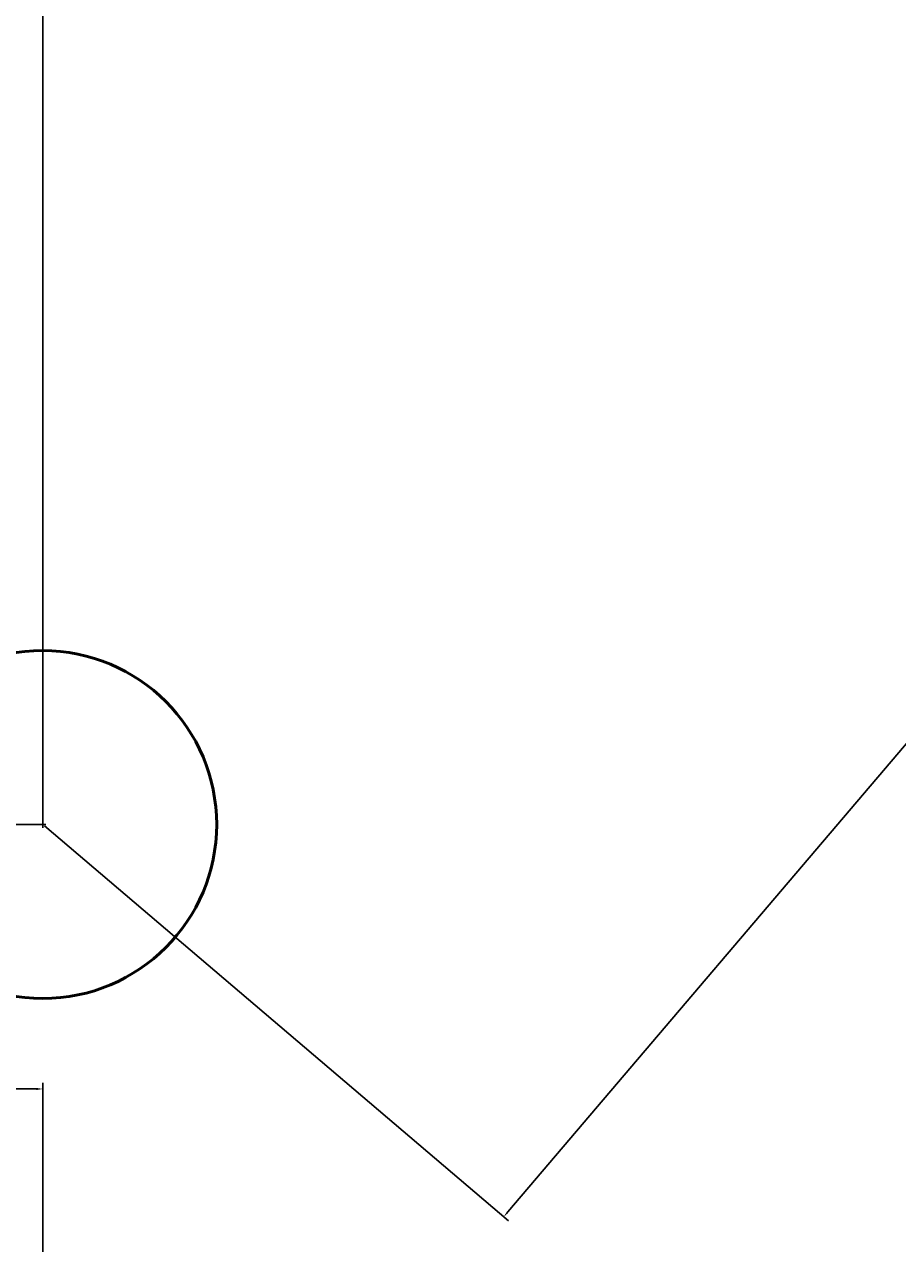
# Model space of a CAD drawing. Units: inches. Extents: x 457 to 775, y 319 to 541.
# Tile 4 of 12: x 554 to 580, y 350 to 385. Entities that reach past the tile are written whole.
import ezdxf

# ---------------------------------------------------------------- set-up
doc = ezdxf.new("R2010")
doc.units = ezdxf.units.IN
doc.header["$MEASUREMENT"] = 0
doc.layers.add('M-DIMS', color=2, linetype='Continuous', lineweight=18)
doc.layers.add('M-OUTL', color=7, linetype='Continuous', lineweight=50)
doc.styles.get("Standard").update_dxf_attribs({"font": 'arial.ttf'})
doc.dimstyles.get("Standard").update_dxf_attribs({"dimtxt": 0.18, "dimasz": 0.18, "dimexe": 0.18, "dimexo": 0.0625, "dimgap": 0.09, "dimtad": 0, "dimtih": 1, "dimtoh": 1, "dimdec": 4, "dimzin": 0, "dimdsep": 46, "dimtxsty": 'Standard', "dimcen": 0.09, "dimadec": 0, "dimazin": 0, "dimtfac": 1, "dimtdec": 4, "dimtofl": 0, "dimtmove": 0, "dimatfit": 3, "dimfxl": 1, "dimtolj": 1, "dimtzin": 0, "dimarcsym": 0})

# ---------------------------------------------------------------- blocks, each defined once
blk = doc.blocks.new('MOUNT-HOLE-D10')
blk.add_circle((5, 5), 5)
blk = doc.blocks.new('*D2')
at = {"layer": 'Defpoints', "color": 0, "transparency": 16777216}
for p in [(756.931, 375.696), (474.306, 336.696), (756.931, 319.296)]:
    blk.add_point(p, dxfattribs=at)
at = {"layer": 'M-DIMS', "color": 0, "lineweight": -2, "transparency": 16777216}
for p, q in [((756.931, 375.634), (756.931, 319.116)), ((474.306, 336.634), (474.306, 319.116)), ((474.486, 319.296), (615.223, 319.296)), ((756.751, 319.296), (616.014, 319.296))]:
    blk.add_line(p, q, dxfattribs=at)
at = {"layer": 'M-DIMS', "color": 0, "transparency": 16777216}
for points in [[(474.486, 319.326), (474.486, 319.266), (474.306, 319.296)], [(756.751, 319.326), (756.751, 319.266), (756.931, 319.296)]]:
    blk.add_solid(points, dxfattribs=at)
at = {"layer": 'M-DIMS', "color": 0, "transparency": 16777216, "insert": (615.619, 319.296), "char_height": 0.18, "attachment_point": 5}
blk.add_mtext('\\A1;282.6', dxfattribs=at)
blk = doc.blocks.new('*D3')
at = {"layer": 'Defpoints', "color": 0, "transparency": 16777216}
for p in [(456.906, 523.213), (646.001, 523.213), (474.306, 336.696)]:
    blk.add_point(p, dxfattribs=at)
at = {"layer": 'M-DIMS', "color": 0, "lineweight": -2, "transparency": 16777216}
for p, q in [((645.939, 523.213), (456.726, 523.213)), ((456.906, 523.033), (456.906, 430.136)), ((456.906, 336.876), (456.906, 429.773)), ((474.244, 336.696), (456.726, 336.696))]:
    blk.add_line(p, q, dxfattribs=at)
at = {"layer": 'M-DIMS', "color": 0, "transparency": 16777216}
for points in [[(456.876, 523.033), (456.936, 523.033), (456.906, 523.213)], [(456.876, 336.876), (456.936, 336.876), (456.906, 336.696)]]:
    blk.add_solid(points, dxfattribs=at)
at = {"layer": 'M-DIMS', "color": 0, "transparency": 16777216, "insert": (456.906, 429.954), "char_height": 0.18, "attachment_point": 5}
blk.add_mtext('\\A1;186.5', dxfattribs=at)
blk = doc.blocks.new('*D6')
at = {"layer": 'Defpoints', "color": 0, "transparency": 16777216}
for p in [(554.931, 354.096), (474.306, 336.696), (554.931, 336.696)]:
    blk.add_point(p, dxfattribs=at)
at = {"layer": 'M-DIMS', "color": 0, "lineweight": -2, "transparency": 16777216}
for p, q in [((474.306, 336.759), (474.306, 354.276)), ((474.486, 354.096), (514.226, 354.096)), ((554.751, 354.096), (515.011, 354.096)), ((554.931, 336.759), (554.931, 354.276))]:
    blk.add_line(p, q, dxfattribs=at)
at = {"layer": 'M-DIMS', "color": 0, "transparency": 16777216}
for points in [[(474.486, 354.126), (474.486, 354.066), (474.306, 354.096)], [(554.751, 354.126), (554.751, 354.066), (554.931, 354.096)]]:
    blk.add_solid(points, dxfattribs=at)
at = {"layer": 'M-DIMS', "color": 0, "transparency": 16777216, "insert": (514.619, 354.096), "char_height": 0.18, "attachment_point": 5}
blk.add_mtext('\\A1;80.62', dxfattribs=at)
blk = doc.blocks.new('*D7')
at = {"layer": 'Defpoints', "color": 0, "transparency": 16777216}
for p in [(537.531, 361.696), (554.931, 361.696), (554.931, 336.696)]:
    blk.add_point(p, dxfattribs=at)
at = {"layer": 'M-DIMS', "color": 0, "lineweight": -2, "transparency": 16777216}
for p, q in [((554.869, 361.696), (537.351, 361.696)), ((537.531, 361.516), (537.531, 349.378)), ((537.531, 336.876), (537.531, 349.014)), ((554.869, 336.696), (537.351, 336.696))]:
    blk.add_line(p, q, dxfattribs=at)
at = {"layer": 'M-DIMS', "color": 0, "transparency": 16777216}
for points in [[(537.501, 361.516), (537.561, 361.516), (537.531, 361.696)], [(537.501, 336.876), (537.561, 336.876), (537.531, 336.696)]]:
    blk.add_solid(points, dxfattribs=at)
at = {"layer": 'M-DIMS', "color": 0, "transparency": 16777216, "insert": (537.531, 349.196), "char_height": 0.18, "attachment_point": 5}
blk.add_mtext('\\A1;25', dxfattribs=at)
blk = doc.blocks.new('*D9')
at = {"layer": 'Defpoints', "color": 0, "transparency": 16777216}
for p in [(756.931, 375.696), (774.331, 375.696), (554.931, 336.696)]:
    blk.add_point(p, dxfattribs=at)
at = {"layer": 'M-DIMS', "color": 0, "lineweight": -2, "transparency": 16777216}
for p, q in [((756.994, 375.696), (774.511, 375.696)), ((774.331, 375.516), (774.331, 356.378)), ((774.331, 336.876), (774.331, 356.014)), ((554.994, 336.696), (774.511, 336.696))]:
    blk.add_line(p, q, dxfattribs=at)
at = {"layer": 'M-DIMS', "color": 0, "transparency": 16777216}
for points in [[(774.301, 375.516), (774.361, 375.516), (774.331, 375.696)], [(774.301, 336.876), (774.361, 336.876), (774.331, 336.696)]]:
    blk.add_solid(points, dxfattribs=at)
at = {"layer": 'M-DIMS', "color": 0, "transparency": 16777216, "insert": (774.331, 356.196), "char_height": 0.18, "attachment_point": 5}
blk.add_mtext('\\A1;39', dxfattribs=at)
blk = doc.blocks.new('*D16')
at = {"layer": 'Defpoints', "color": 0, "transparency": 16777216}
for p in [(554.931, 540.613), (514.502, 430.729), (554.931, 361.696)]:
    blk.add_point(p, dxfattribs=at)
at = {"layer": 'M-DIMS', "color": 0, "lineweight": -2, "transparency": 16777216}
for p, q in [((514.502, 430.791), (514.502, 540.793)), ((554.931, 361.759), (554.931, 540.793)), ((514.682, 540.613), (534.319, 540.613)), ((554.751, 540.613), (535.114, 540.613))]:
    blk.add_line(p, q, dxfattribs=at)
at = {"layer": 'M-DIMS', "color": 0, "transparency": 16777216}
for points in [[(514.682, 540.643), (514.682, 540.583), (514.502, 540.613)], [(554.751, 540.643), (554.751, 540.583), (554.931, 540.613)]]:
    blk.add_solid(points, dxfattribs=at)
at = {"layer": 'M-DIMS', "color": 0, "transparency": 16777216, "insert": (534.716, 540.613), "char_height": 0.18, "attachment_point": 5}
blk.add_mtext('\\A1;40.43', dxfattribs=at)
blk = doc.blocks.new('*D17')
at = {"layer": 'Defpoints', "color": 0, "transparency": 16777216}
for p in [(606.761, 540.613), (606.761, 422.636), (554.931, 361.696)]:
    blk.add_point(p, dxfattribs=at)
at = {"layer": 'M-DIMS', "color": 0, "lineweight": -2, "transparency": 16777216}
for p, q in [((554.931, 361.759), (554.931, 540.793)), ((606.761, 422.698), (606.761, 540.793)), ((555.111, 540.613), (580.452, 540.613)), ((606.581, 540.613), (581.24, 540.613))]:
    blk.add_line(p, q, dxfattribs=at)
at = {"layer": 'M-DIMS', "color": 0, "transparency": 16777216}
for points in [[(555.111, 540.643), (555.111, 540.583), (554.931, 540.613)], [(606.581, 540.643), (606.581, 540.583), (606.761, 540.613)]]:
    blk.add_solid(points, dxfattribs=at)
at = {"layer": 'M-DIMS', "color": 0, "transparency": 16777216, "insert": (580.846, 540.613), "char_height": 0.18, "attachment_point": 5}
blk.add_mtext('\\A1;51.83', dxfattribs=at)
blk = doc.blocks.new('*D18')
at = {"layer": 'Defpoints', "color": 0, "transparency": 16777216}
for p in [(606.761, 422.636), (554.931, 361.696), (568.185, 350.423)]:
    blk.add_point(p, dxfattribs=at)
at = {"layer": 'M-DIMS', "color": 0, "lineweight": -2, "transparency": 16777216}
for p, q in [((606.809, 422.595), (620.153, 411.246)), ((619.899, 411.226), (594.255, 381.075)), ((568.302, 350.56), (593.946, 380.711)), ((554.979, 361.656), (568.323, 350.306))]:
    blk.add_line(p, q, dxfattribs=at)
at = {"layer": 'M-DIMS', "color": 0, "transparency": 16777216}
for points in [[(619.876, 411.245), (619.922, 411.206), (620.015, 411.363)], [(568.279, 350.58), (568.325, 350.541), (568.185, 350.423)]]:
    blk.add_solid(points, dxfattribs=at)
at = {"layer": 'M-DIMS', "color": 0, "transparency": 16777216, "insert": (594.1, 380.893), "char_height": 0.18, "attachment_point": 5}
blk.add_mtext('\\A1;80', dxfattribs=at)
blk = doc.blocks.new('*D19')
at = {"layer": 'Defpoints', "color": 0, "transparency": 16777216}
for p in [(562.393, 446.769), (554.931, 361.696)]:
    blk.add_point(p, dxfattribs=at)
at = {"layer": 'M-DIMS', "color": 0, "lineweight": -2, "transparency": 16777216}
for p, q in [((566.87, 497.813), (562.409, 446.949)), ((567.05, 497.813), (566.87, 497.813)), ((554.841, 361.696), (555.021, 361.696)), ((554.931, 361.606), (554.931, 361.786))]:
    blk.add_line(p, q, dxfattribs=at)
at = {"layer": 'M-DIMS', "color": 0, "transparency": 16777216}
blk.add_solid([(562.379, 446.951), (562.439, 446.946), (562.393, 446.769)], dxfattribs=at)
at = {"layer": 'M-DIMS', "color": 0, "transparency": 16777216, "insert": (567.46, 497.813), "char_height": 0.18, "attachment_point": 5}
blk.add_mtext('\\A1;R85.4', dxfattribs=at)
blk = doc.blocks.new('*D20')
at = {"layer": 'Defpoints', "color": 0, "transparency": 16777216}
for p in [(561.45, 436.011), (554.931, 361.696)]:
    blk.add_point(p, dxfattribs=at)
at = {"layer": 'M-DIMS', "color": 0, "lineweight": -2, "transparency": 16777216}
for p, q in [((565.361, 480.599), (561.466, 436.19)), ((565.541, 480.599), (565.361, 480.599)), ((554.841, 361.696), (555.021, 361.696)), ((554.931, 361.606), (554.931, 361.786))]:
    blk.add_line(p, q, dxfattribs=at)
at = {"layer": 'M-DIMS', "color": 0, "transparency": 16777216}
blk.add_solid([(561.436, 436.193), (561.496, 436.187), (561.45, 436.011)], dxfattribs=at)
at = {"layer": 'M-DIMS', "color": 0, "transparency": 16777216, "insert": (565.951, 480.599), "char_height": 0.18, "attachment_point": 5}
blk.add_mtext('\\A1;R74.6', dxfattribs=at)

msp = doc.modelspace()

# ---------------------------------------------------------------- block references
at = {"layer": 'M-OUTL'}
msp.add_blockref('MOUNT-HOLE-D10', (549.931, 356.696), dxfattribs=at)

# ---------------------------------------------------------------- dimensions: what is measured, and where the dimension line sits
at = {"layer": 'M-DIMS'}
for base, p1, p2, override, picture, middle in [((554.931, 540.613), (514.502, 430.729), (554.931, 361.696), {"dimdec": 2, "dimlfac": 1, "dimrnd": 0, "dimzin": 0, "dimdsep": 46, "dimlunit": 2}, '*D16', (534.716, 540.613)), ((606.761, 540.613), (554.931, 361.696), (606.761, 422.636), {"dimdec": 2, "dimlfac": 1, "dimrnd": 0, "dimzin": 0, "dimdsep": 46, "dimlunit": 2}, '*D17', (580.846, 540.613)), ((756.931, 319.296), (474.306, 336.696), (756.931, 375.696), {"dimdec": 1, "dimlfac": 1, "dimrnd": 0, "dimzin": 0, "dimdsep": 46, "dimlunit": 2}, '*D2', (615.619, 319.296)), ((554.931, 354.096), (474.3061, 336.696), (554.931, 336.696), {"dimdec": 2, "dimlfac": 1, "dimrnd": 0, "dimzin": 0, "dimdsep": 46, "dimlunit": 2}, '*D6', (514.6186, 354.096))]:
    dim = msp.add_linear_dim(base=base, p1=p1, p2=p2, dimstyle='Standard', override=override, dxfattribs=at)
    dim.commit()
    dim.dimension.update_dxf_attribs({"geometry": picture, "text_midpoint": middle})
for base, p1, p2, angle, override, picture, middle in [((456.906, 523.213), (474.306, 336.696), (646.001, 523.213), 90, {"dimdec": 1, "dimlfac": 1, "dimrnd": 0, "dimzin": 0, "dimdsep": 46, "dimlunit": 2}, '*D3', (456.906, 429.954)), ((568.185, 350.423), (606.761, 422.636), (554.931, 361.696), 229.6185, {"dimdec": 0, "dimlfac": 1, "dimrnd": 0, "dimzin": 0, "dimdsep": 46, "dimlunit": 2}, '*D18', (594.1, 380.893)), ((774.331, 375.696), (554.931, 336.696), (756.931, 375.696), 90, {"dimdec": 0, "dimlfac": 1, "dimrnd": 0, "dimzin": 0, "dimdsep": 46, "dimlunit": 2}, '*D9', (774.331, 356.196)), ((537.531, 361.696), (554.931, 336.696), (554.931, 361.696), 90, {"dimdec": 0, "dimlfac": 1, "dimrnd": 0, "dimzin": 0, "dimdsep": 46, "dimlunit": 2}, '*D7', (537.531, 349.196))]:
    dim = msp.add_linear_dim(base=base, p1=p1, p2=p2, angle=angle, dimstyle='Standard', override=override, dxfattribs=at)
    dim.commit()
    dim.dimension.update_dxf_attribs({"geometry": picture, "text_midpoint": middle})
for mpoint, picture, middle in [((562.393, 446.769), '*D19', (567.46, 497.813)), ((561.45, 436.011), '*D20', (565.951, 480.599))]:
    dim = msp.add_radius_dim(center=(554.931, 361.696), mpoint=mpoint, dimstyle='Standard', override={"dimdec": 1, "dimlfac": 1, "dimrnd": 0, "dimzin": 0, "dimdsep": 46, "dimlunit": 2}, dxfattribs=at)
    dim.commit()
    dim.dimension.update_dxf_attribs({"geometry": picture, "text_midpoint": middle, "dimtype": 164})

doc.saveas('drawing.dxf')
